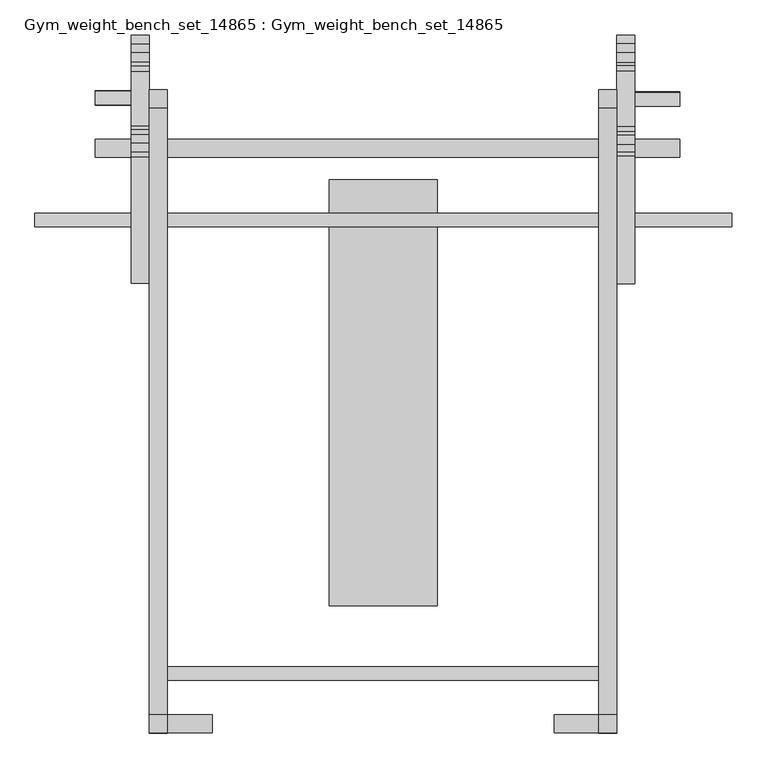
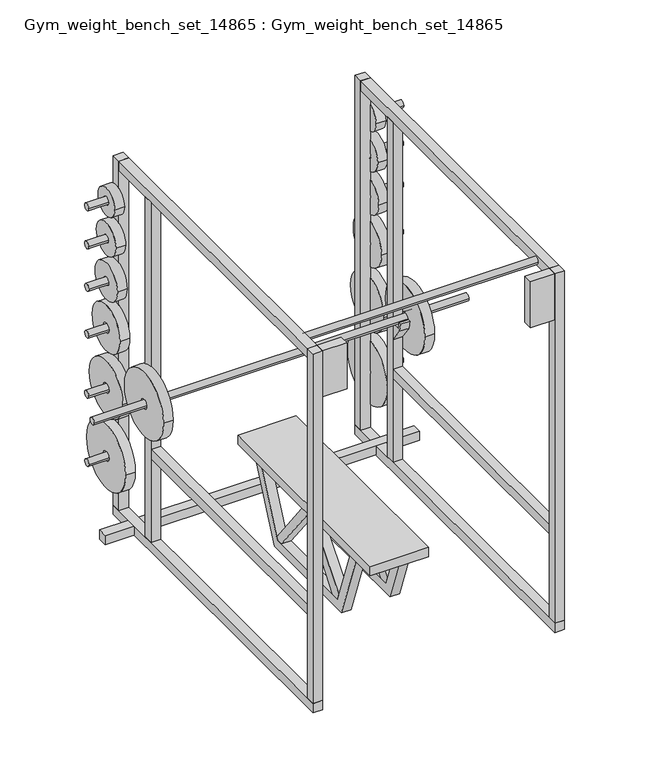
"""IFC4 building model written with IfcOpenShell, lengths in millimetres: furniture geometry, Gym_weight_bench_set_14865 : Gym_weight_bench_set_14865."""

from ifc_helpers import new_model, si_unit, point, frame, frame_2d, origin, place, context, project, spatial, polyline, circle_curve, trimmed, segment, composite_curve, outline, extrude, source, transform, mapped, element, save


def gym_weight_bench_set_14865_gym_weight_bench_set_14865_0f5544b4(model_context):
    return source(origin(), model_context, "Body", "SweptSolid", [
        extrude(outline(polyline([(0.0, 1816.1), (50.8, 1816.1), (50.8, 0.0), (0.0, 0.0), (0.0, 1816.1)])), frame((0.0, 0.0, 93.2100633), z_axis=(0.0, 0.0, 1.0), x_axis=(1.0, 0.0, 0.0)), (0.0, 0.0, 1.0), 50.8),
        extrude(outline(polyline([(0.0, 0.0), (0.0, 50.8), (50.8, 50.8), (50.8, 0.0), (0.0, 0.0)])), frame((0.0, 0.0, 144.0100633), z_axis=(0.0, 0.0, 1.0), x_axis=(1.0, 0.0, 0.0)), (0.0, 0.0, 1.0), 1938.7899367),
        extrude(outline(polyline([(0.0, 1473.2), (0.0, 1524.0), (50.8, 1524.0), (50.8, 1473.2), (0.0, 1473.2)])), frame((0.0, 0.0, 144.0100633), z_axis=(0.0, 0.0, 1.0), x_axis=(1.0, 0.0, 0.0)), (0.0, 0.0, 1.0), 1887.9899367),
        extrude(outline(polyline([(-152.4, 1676.4), (0.0, 1676.4), (50.8, 1676.4), (1270.0, 1676.4), (1498.6, 1676.4), (1498.6, 1625.6), (-152.4, 1625.6), (-152.4, 1676.4)])), frame((0.0, 0.0, 93.2100633), z_axis=(0.0, 0.0, 1.0), x_axis=(1.0, 0.0, 0.0)), (0.0, 0.0, 1.0), 50.8),
        extrude(outline(polyline([(1270.0, 1816.1), (1320.8, 1816.1), (1320.8, 0.0), (1270.0, 0.0), (1270.0, 1816.1)])), frame((0.0, 0.0, 93.2100633), z_axis=(0.0, 0.0, 1.0), x_axis=(1.0, 0.0, 0.0)), (0.0, 0.0, 1.0), 50.8),
        extrude(outline(polyline([(1270.0, 0.0), (1270.0, 50.8), (1320.8, 50.8), (1320.8, 0.0), (1270.0, 0.0)])), frame((0.0, 0.0, 144.0100633), z_axis=(0.0, 0.0, 1.0), x_axis=(1.0, 0.0, 0.0)), (0.0, 0.0, 1.0), 1938.7899367),
        extrude(outline(polyline([(1270.0, 1473.2), (1270.0, 1524.0), (1320.8, 1524.0), (1320.8, 1473.2), (1270.0, 1473.2)])), frame((0.0, 0.0, 144.0100633), z_axis=(0.0, 0.0, 1.0), x_axis=(1.0, 0.0, 0.0)), (0.0, 0.0, 1.0), 1887.9899367),
        extrude(outline(polyline([(0.0, 1765.3), (0.0, 1816.1), (50.8, 1816.1), (50.8, 1765.3), (0.0, 1765.3)])), frame((0.0, 0.0, 144.0100633), z_axis=(0.0, 0.0, 1.0), x_axis=(1.0, 0.0, 0.0)), (0.0, 0.0, 1.0), 1938.7899367),
        extrude(outline(polyline([(1270.0, 1765.3), (1270.0, 1816.1), (1320.8, 1816.1), (1320.8, 1765.3), (1270.0, 1765.3)])), frame((0.0, 0.0, 144.0100633), z_axis=(0.0, 0.0, 1.0), x_axis=(1.0, 0.0, 0.0)), (0.0, 0.0, 1.0), 1938.7899367),
        extrude(outline(polyline([(0.0, 50.8), (0.0, 1816.1), (50.8, 1816.1), (50.8, 50.8), (0.0, 50.8)])), frame((0.0, 0.0, 2032.0), z_axis=(0.0, 0.0, 1.0), x_axis=(1.0, 0.0, 0.0)), (0.0, 0.0, 1.0), 50.8),
        extrude(outline(polyline([(1270.0, 50.8), (1270.0, 1816.1), (1320.8, 1816.1), (1320.8, 50.8), (1270.0, 50.8)])), frame((0.0, 0.0, 2032.0), z_axis=(0.0, 0.0, 1.0), x_axis=(1.0, 0.0, 0.0)), (0.0, 0.0, 1.0), 50.8),
        extrude(outline(polyline([(0.0, 50.8), (0.0, 1473.2), (50.8, 1473.2), (50.8, 50.8), (0.0, 50.8)])), frame((0.0, 0.0, 609.6), z_axis=(0.0, 0.0, 1.0), x_axis=(1.0, 0.0, 0.0)), (0.0, 0.0, 1.0), 50.8),
        extrude(outline(polyline([(1270.0, 50.8), (1270.0, 1473.2), (1320.8, 1473.2), (1320.8, 50.8), (1270.0, 50.8)])), frame((0.0, 0.0, 609.6), z_axis=(0.0, 0.0, 1.0), x_axis=(1.0, 0.0, 0.0)), (0.0, 0.0, 1.0), 50.8),
        extrude(outline(composite_curve([segment(trimmed(circle_curve(frame_2d((168.0556142, 2057.8602895)), 19.05), [point((149.0056142, 2057.8602895))], [point((187.1056142, 2057.8602895))], False, "CARTESIAN"), True, "CONTINUOUS"), segment(trimmed(circle_curve(frame_2d((168.0556142, 2057.8602895)), 19.05), [point((187.1056142, 2057.8602895))], [point((149.0056142, 2057.8602895))], False, "CARTESIAN"), True, "CONTINUOUS")], self_intersect=False)), frame((50.8, 0.0, 0.0), z_axis=(1.0, 0.0, 0.0), x_axis=(0.0, 1.0, 0.0)), (0.0, 0.0, 1.0), 1219.2),
        extrude(outline(composite_curve([segment(trimmed(circle_curve(frame_2d((1791.2245511, 448.53524)), 19.05), [point((1772.1745511, 448.53524))], [point((1810.2745511, 448.53524))], False, "CARTESIAN"), True, "CONTINUOUS"), segment(trimmed(circle_curve(frame_2d((1791.2245511, 448.53524)), 19.05), [point((1810.2745511, 448.53524))], [point((1772.1745511, 448.53524))], False, "CARTESIAN"), True, "CONTINUOUS")], self_intersect=False)), frame((-152.4, 0.0, 0.0), z_axis=(1.0, 0.0, 0.0), x_axis=(0.0, 1.0, 0.0)), (0.0, 0.0, 1.0), 152.4),
        extrude(outline(composite_curve([segment(trimmed(circle_curve(frame_2d((1792.8120511, 826.36024)), 19.05), [point((1773.7620511, 826.36024))], [point((1811.8620511, 826.36024))], False, "CARTESIAN"), True, "CONTINUOUS"), segment(trimmed(circle_curve(frame_2d((1792.8120511, 826.36024)), 19.05), [point((1811.8620511, 826.36024))], [point((1773.7620511, 826.36024))], False, "CARTESIAN"), True, "CONTINUOUS")], self_intersect=False)), frame((-152.4, 0.0, 0.0), z_axis=(1.0, 0.0, 0.0), x_axis=(0.0, 1.0, 0.0)), (0.0, 0.0, 1.0), 152.4),
        extrude(outline(composite_curve([segment(trimmed(circle_curve(frame_2d((1792.4151761, 1865.775865)), 19.05), [point((1773.3651761, 1865.775865))], [point((1811.4651761, 1865.775865))], False, "CARTESIAN"), True, "CONTINUOUS"), segment(trimmed(circle_curve(frame_2d((1792.4151761, 1865.775865)), 19.05), [point((1811.4651761, 1865.775865))], [point((1773.3651761, 1865.775865))], False, "CARTESIAN"), True, "CONTINUOUS")], self_intersect=False)), frame((-152.4, 0.0, 0.0), z_axis=(1.0, 0.0, 0.0), x_axis=(0.0, 1.0, 0.0)), (0.0, 0.0, 1.0), 152.4),
        extrude(outline(composite_curve([segment(trimmed(circle_curve(frame_2d((1793.6058011, 1654.24149)), 19.05), [point((1774.5558011, 1654.24149))], [point((1812.6558011, 1654.24149))], False, "CARTESIAN"), True, "CONTINUOUS"), segment(trimmed(circle_curve(frame_2d((1793.6058011, 1654.24149)), 19.05), [point((1812.6558011, 1654.24149))], [point((1774.5558011, 1654.24149))], False, "CARTESIAN"), True, "CONTINUOUS")], self_intersect=False)), frame((-152.4, 0.0, 0.0), z_axis=(1.0, 0.0, 0.0), x_axis=(0.0, 1.0, 0.0)), (0.0, 0.0, 1.0), 152.4),
        extrude(outline(composite_curve([segment(trimmed(circle_curve(frame_2d((1791.2245511, 1420.08524)), 19.05), [point((1772.1745511, 1420.08524))], [point((1810.2745511, 1420.08524))], False, "CARTESIAN"), True, "CONTINUOUS"), segment(trimmed(circle_curve(frame_2d((1791.2245511, 1420.08524)), 19.05), [point((1810.2745511, 1420.08524))], [point((1772.1745511, 1420.08524))], False, "CARTESIAN"), True, "CONTINUOUS")], self_intersect=False)), frame((-152.4, 0.0, 0.0), z_axis=(1.0, 0.0, 0.0), x_axis=(0.0, 1.0, 0.0)), (0.0, 0.0, 1.0), 152.4),
        extrude(outline(composite_curve([segment(trimmed(circle_curve(frame_2d((1792.0183011, 1159.73524)), 19.05), [point((1772.9683011, 1159.73524))], [point((1811.0683011, 1159.73524))], False, "CARTESIAN"), True, "CONTINUOUS"), segment(trimmed(circle_curve(frame_2d((1792.0183011, 1159.73524)), 19.05), [point((1811.0683011, 1159.73524))], [point((1772.9683011, 1159.73524))], False, "CARTESIAN"), True, "CONTINUOUS")], self_intersect=False)), frame((-152.4, 0.0, 0.0), z_axis=(1.0, 0.0, 0.0), x_axis=(0.0, 1.0, 0.0)), (0.0, 0.0, 1.0), 152.4),
        extrude(outline(composite_curve([segment(trimmed(circle_curve(frame_2d((1788.3835299, 1862.6771224)), 19.05), [point((1769.3335299, 1862.6771224))], [point((1807.4335299, 1862.6771224))], False, "CARTESIAN"), True, "CONTINUOUS"), segment(trimmed(circle_curve(frame_2d((1788.3835299, 1862.6771224)), 19.05), [point((1807.4335299, 1862.6771224))], [point((1769.3335299, 1862.6771224))], False, "CARTESIAN"), True, "CONTINUOUS")], self_intersect=False)), frame((1320.8, 0.0, 0.0), z_axis=(1.0, 0.0, 0.0), x_axis=(0.0, 1.0, 0.0)), (0.0, 0.0, 1.0), 177.8),
        extrude(outline(composite_curve([segment(trimmed(circle_curve(frame_2d((1789.9710299, 1650.9298353)), 19.05), [point((1770.9210299, 1650.9298353))], [point((1809.0210299, 1650.9298353))], False, "CARTESIAN"), True, "CONTINUOUS"), segment(trimmed(circle_curve(frame_2d((1789.9710299, 1650.9298353)), 19.05), [point((1809.0210299, 1650.9298353))], [point((1770.9210299, 1650.9298353))], False, "CARTESIAN"), True, "CONTINUOUS")], self_intersect=False)), frame((1320.8, 0.0, 0.0), z_axis=(1.0, 0.0, 0.0), x_axis=(0.0, 1.0, 0.0)), (0.0, 0.0, 1.0), 177.8),
        extrude(outline(composite_curve([segment(trimmed(circle_curve(frame_2d((1789.9710299, 1422.3298353)), 19.05), [point((1770.9210299, 1422.3298353))], [point((1809.0210299, 1422.3298353))], False, "CARTESIAN"), True, "CONTINUOUS"), segment(trimmed(circle_curve(frame_2d((1789.9710299, 1422.3298353)), 19.05), [point((1809.0210299, 1422.3298353))], [point((1770.9210299, 1422.3298353))], False, "CARTESIAN"), True, "CONTINUOUS")], self_intersect=False)), frame((1320.8, 0.0, 0.0), z_axis=(1.0, 0.0, 0.0), x_axis=(0.0, 1.0, 0.0)), (0.0, 0.0, 1.0), 177.8),
        extrude(outline(composite_curve([segment(trimmed(circle_curve(frame_2d((1789.9710299, 1160.2424636)), 19.05), [point((1770.9210299, 1160.2424636))], [point((1809.0210299, 1160.2424636))], False, "CARTESIAN"), True, "CONTINUOUS"), segment(trimmed(circle_curve(frame_2d((1789.9710299, 1160.2424636)), 19.05), [point((1809.0210299, 1160.2424636))], [point((1770.9210299, 1160.2424636))], False, "CARTESIAN"), True, "CONTINUOUS")], self_intersect=False)), frame((1320.8, 0.0, 0.0), z_axis=(1.0, 0.0, 0.0), x_axis=(0.0, 1.0, 0.0)), (0.0, 0.0, 1.0), 177.8),
        extrude(outline(composite_curve([segment(trimmed(circle_curve(frame_2d((1791.5585299, 826.8674636)), 19.05), [point((1772.5085299, 826.8674636))], [point((1810.6085299, 826.8674636))], False, "CARTESIAN"), True, "CONTINUOUS"), segment(trimmed(circle_curve(frame_2d((1791.5585299, 826.8674636)), 19.05), [point((1810.6085299, 826.8674636))], [point((1772.5085299, 826.8674636))], False, "CARTESIAN"), True, "CONTINUOUS")], self_intersect=False)), frame((1320.8, 0.0, 0.0), z_axis=(1.0, 0.0, 0.0), x_axis=(0.0, 1.0, 0.0)), (0.0, 0.0, 1.0), 177.8),
        extrude(outline(composite_curve([segment(trimmed(circle_curve(frame_2d((1789.9710299, 448.917051)), 19.05), [point((1770.9210299, 448.917051))], [point((1809.0210299, 448.917051))], False, "CARTESIAN"), True, "CONTINUOUS"), segment(trimmed(circle_curve(frame_2d((1789.9710299, 448.917051)), 19.05), [point((1809.0210299, 448.917051))], [point((1770.9210299, 448.917051))], False, "CARTESIAN"), True, "CONTINUOUS")], self_intersect=False)), frame((1320.8, 0.0, 0.0), z_axis=(1.0, 0.0, 0.0), x_axis=(0.0, 1.0, 0.0)), (0.0, 0.0, 1.0), 177.8),
        extrude(outline(polyline([(177.8, 0.0), (50.8, 0.0), (50.8, 50.8), (177.8, 50.8), (177.8, 0.0)])), frame((0.0, 0.0, 1828.8), z_axis=(0.0, 0.0, 1.0), x_axis=(1.0, 0.0, 0.0)), (0.0, 0.0, 1.0), 254.0),
        extrude(outline(polyline([(1270.0, 0.0), (1143.0, 0.0), (1143.0, 50.8), (1270.0, 50.8), (1270.0, 0.0)])), frame((0.0, 0.0, 1828.8), z_axis=(0.0, 0.0, 1.0), x_axis=(1.0, 0.0, 0.0)), (0.0, 0.0, 1.0), 254.0),
        extrude(outline(composite_curve([segment(trimmed(circle_curve(frame_2d((1448.5134797, 945.953956)), 19.05), [point((1429.4634797, 945.953956))], [point((1467.5634797, 945.953956))], False, "CARTESIAN"), True, "CONTINUOUS"), segment(trimmed(circle_curve(frame_2d((1448.5134797, 945.953956)), 19.05), [point((1467.5634797, 945.953956))], [point((1429.4634797, 945.953956))], False, "CARTESIAN"), True, "CONTINUOUS")], self_intersect=False)), frame((-322.3423226, 0.0, 0.0), z_axis=(1.0, 0.0, 0.0), x_axis=(0.0, 1.0, 0.0)), (0.0, 0.0, 1.0), 1966.9449532),
        extrude(outline(polyline([(1422.4, 920.0682148), (1473.2, 920.0682148), (1473.2, 823.1962833), (1411.9053319, 907.5611564), (1404.1016184, 951.8182148), (1416.8016184, 951.8182148), (1422.4, 920.0682148)])), frame((0.0, 0.0, 0.0), z_axis=(1.0, 0.0, 0.0), x_axis=(0.0, 1.0, 0.0)), (0.0, 0.0, 1.0), 50.8),
        extrude(outline(polyline([(1422.4, 920.0682148), (1473.2, 920.0682148), (1473.2, 823.1962833), (1411.9053319, 907.5611564), (1404.1016184, 951.8182148), (1416.8016184, 951.8182148), (1422.4, 920.0682148)])), frame((1270.0, 0.0, 0.0), z_axis=(1.0, 0.0, 0.0), x_axis=(0.0, 1.0, 0.0)), (0.0, 0.0, 1.0), 50.8),
        extrude(outline(composite_curve([segment(trimmed(circle_curve(frame_2d((1792.6730331, 448.4299911)), 177.8), [point((1614.8730331, 448.4299911))], [point((1970.4730331, 448.4299911))], False, "CARTESIAN"), True, "CONTINUOUS"), segment(trimmed(circle_curve(frame_2d((1792.6730331, 448.4299911)), 177.8), [point((1970.4730331, 448.4299911))], [point((1614.8730331, 448.4299911))], False, "CARTESIAN"), True, "CONTINUOUS")], self_intersect=False), holes=[composite_curve([segment(trimmed(circle_curve(frame_2d((1792.6730331, 448.4299911)), 25.7855331), [point((1766.8875, 448.4299911))], [point((1818.4585662, 448.4299911))], True, "CARTESIAN"), True, "CONTINUOUS"), segment(trimmed(circle_curve(frame_2d((1792.6730331, 448.4299911)), 25.7855331), [point((1818.4585662, 448.4299911))], [point((1766.8875, 448.4299911))], True, "CARTESIAN"), True, "CONTINUOUS")], self_intersect=False)]), frame((-50.8, 0.0, 0.0), z_axis=(1.0, 0.0, 0.0), x_axis=(0.0, 1.0, 0.0)), (0.0, 0.0, 1.0), 50.8),
        extrude(outline(composite_curve([segment(trimmed(circle_curve(frame_2d((1792.6730331, 826.2549911)), 152.4), [point((1640.2730331, 826.2549911))], [point((1945.0730331, 826.2549911))], False, "CARTESIAN"), True, "CONTINUOUS"), segment(trimmed(circle_curve(frame_2d((1792.6730331, 826.2549911)), 152.4), [point((1945.0730331, 826.2549911))], [point((1640.2730331, 826.2549911))], False, "CARTESIAN"), True, "CONTINUOUS")], self_intersect=False), holes=[composite_curve([segment(trimmed(circle_curve(frame_2d((1792.6730331, 826.2549911)), 25.7855331), [point((1766.8875, 826.2549911))], [point((1818.4585662, 826.2549911))], True, "CARTESIAN"), True, "CONTINUOUS"), segment(trimmed(circle_curve(frame_2d((1792.6730331, 826.2549911)), 25.7855331), [point((1818.4585662, 826.2549911))], [point((1766.8875, 826.2549911))], True, "CARTESIAN"), True, "CONTINUOUS")], self_intersect=False)]), frame((-50.8, 0.0, 0.0), z_axis=(1.0, 0.0, 0.0), x_axis=(0.0, 1.0, 0.0)), (0.0, 0.0, 1.0), 50.8),
        extrude(outline(composite_curve([segment(trimmed(circle_curve(frame_2d((1792.6730331, 1159.6299911)), 127.0), [point((1665.6730331, 1159.6299911))], [point((1919.6730331, 1159.6299911))], False, "CARTESIAN"), True, "CONTINUOUS"), segment(trimmed(circle_curve(frame_2d((1792.6730331, 1159.6299911)), 127.0), [point((1919.6730331, 1159.6299911))], [point((1665.6730331, 1159.6299911))], False, "CARTESIAN"), True, "CONTINUOUS")], self_intersect=False), holes=[composite_curve([segment(trimmed(circle_curve(frame_2d((1792.6730331, 1159.6299911)), 25.7855331), [point((1766.8875, 1159.6299911))], [point((1818.4585662, 1159.6299911))], True, "CARTESIAN"), True, "CONTINUOUS"), segment(trimmed(circle_curve(frame_2d((1792.6730331, 1159.6299911)), 25.7855331), [point((1818.4585662, 1159.6299911))], [point((1766.8875, 1159.6299911))], True, "CARTESIAN"), True, "CONTINUOUS")], self_intersect=False)]), frame((-50.8, 0.0, 0.0), z_axis=(1.0, 0.0, 0.0), x_axis=(0.0, 1.0, 0.0)), (0.0, 0.0, 1.0), 50.8),
        extrude(outline(composite_curve([segment(trimmed(circle_curve(frame_2d((1448.1855331, 945.5372652)), 177.8), [point((1270.3855331, 945.5372652))], [point((1625.9855331, 945.5372652))], False, "CARTESIAN"), True, "CONTINUOUS"), segment(trimmed(circle_curve(frame_2d((1448.1855331, 945.5372652)), 177.8), [point((1625.9855331, 945.5372652))], [point((1270.3855331, 945.5372652))], False, "CARTESIAN"), True, "CONTINUOUS")], self_intersect=False), holes=[composite_curve([segment(trimmed(circle_curve(frame_2d((1448.1855331, 945.5372652)), 25.7855331), [point((1422.4, 945.5372652))], [point((1473.9710662, 945.5372652))], True, "CARTESIAN"), True, "CONTINUOUS"), segment(trimmed(circle_curve(frame_2d((1448.1855331, 945.5372652)), 25.7855331), [point((1473.9710662, 945.5372652))], [point((1422.4, 945.5372652))], True, "CARTESIAN"), True, "CONTINUOUS")], self_intersect=False)]), frame((-50.8, 0.0, 0.0), z_axis=(1.0, 0.0, 0.0), x_axis=(0.0, 1.0, 0.0)), (0.0, 0.0, 1.0), 50.8),
        extrude(outline(composite_curve([segment(trimmed(circle_curve(frame_2d((1790.3721267, 1859.8407645)), 76.2), [point((1714.1721267, 1859.8407645))], [point((1866.5721267, 1859.8407645))], False, "CARTESIAN"), True, "CONTINUOUS"), segment(trimmed(circle_curve(frame_2d((1790.3721267, 1859.8407645)), 76.2), [point((1866.5721267, 1859.8407645))], [point((1714.1721267, 1859.8407645))], False, "CARTESIAN"), True, "CONTINUOUS")], self_intersect=False), holes=[composite_curve([segment(trimmed(circle_curve(frame_2d((1792.2369373, 1865.5999932)), 21.4432675), [point((1770.7936698, 1865.5999932))], [point((1813.6802049, 1865.5999932))], True, "CARTESIAN"), True, "CONTINUOUS"), segment(trimmed(circle_curve(frame_2d((1792.2369373, 1865.5999932)), 21.4432675), [point((1813.6802049, 1865.5999932))], [point((1770.7936698, 1865.5999932))], True, "CARTESIAN"), True, "CONTINUOUS")], self_intersect=False)]), frame((-50.8, 0.0, 0.0), z_axis=(1.0, 0.0, 0.0), x_axis=(0.0, 1.0, 0.0)), (0.0, 0.0, 1.0), 50.8),
        extrude(outline(composite_curve([segment(trimmed(circle_curve(frame_2d((1792.64404, 1654.3866671)), 88.9), [point((1703.74404, 1654.3866671))], [point((1881.54404, 1654.3866671))], False, "CARTESIAN"), True, "CONTINUOUS"), segment(trimmed(circle_curve(frame_2d((1792.64404, 1654.3866671)), 88.9), [point((1881.54404, 1654.3866671))], [point((1703.74404, 1654.3866671))], False, "CARTESIAN"), True, "CONTINUOUS")], self_intersect=False), holes=[composite_curve([segment(trimmed(circle_curve(frame_2d((1792.64404, 1654.3866671)), 20.7181506), [point((1771.9258894, 1654.3866671))], [point((1813.3621906, 1654.3866671))], True, "CARTESIAN"), True, "CONTINUOUS"), segment(trimmed(circle_curve(frame_2d((1792.64404, 1654.3866671)), 20.7181506), [point((1813.3621906, 1654.3866671))], [point((1771.9258894, 1654.3866671))], True, "CARTESIAN"), True, "CONTINUOUS")], self_intersect=False)]), frame((-50.8, 0.0, 0.0), z_axis=(1.0, 0.0, 0.0), x_axis=(0.0, 1.0, 0.0)), (0.0, 0.0, 1.0), 50.8),
        extrude(outline(composite_curve([segment(trimmed(circle_curve(frame_2d((1791.2896953, 1420.0850266)), 101.6), [point((1689.6896953, 1420.0850266))], [point((1892.8896953, 1420.0850266))], False, "CARTESIAN"), True, "CONTINUOUS"), segment(trimmed(circle_curve(frame_2d((1791.2896953, 1420.0850266)), 101.6), [point((1892.8896953, 1420.0850266))], [point((1689.6896953, 1420.0850266))], False, "CARTESIAN"), True, "CONTINUOUS")], self_intersect=False), holes=[composite_curve([segment(trimmed(circle_curve(frame_2d((1791.2896953, 1420.0850266)), 21.3349156), [point((1769.9547796, 1420.0850266))], [point((1812.6246109, 1420.0850266))], True, "CARTESIAN"), True, "CONTINUOUS"), segment(trimmed(circle_curve(frame_2d((1791.2896953, 1420.0850266)), 21.3349156), [point((1812.6246109, 1420.0850266))], [point((1769.9547796, 1420.0850266))], True, "CARTESIAN"), True, "CONTINUOUS")], self_intersect=False)]), frame((-50.8, 0.0, 0.0), z_axis=(1.0, 0.0, 0.0), x_axis=(0.0, 1.0, 0.0)), (0.0, 0.0, 1.0), 50.8),
        extrude(outline(composite_curve([segment(trimmed(circle_curve(frame_2d((1791.0047799, 449.3731485)), 179.5423329), [point((1611.462447, 449.3731485))], [point((1970.5471128, 449.3731485))], False, "CARTESIAN"), True, "CONTINUOUS"), segment(trimmed(circle_curve(frame_2d((1791.0047799, 449.3731485)), 179.5423329), [point((1970.5471128, 449.3731485))], [point((1611.462447, 449.3731485))], False, "CARTESIAN"), True, "CONTINUOUS")], self_intersect=False), holes=[composite_curve([segment(trimmed(circle_curve(frame_2d((1791.0047799, 449.3731485)), 25.9804836), [point((1765.0242963, 449.3731485))], [point((1816.9852635, 449.3731485))], True, "CARTESIAN"), True, "CONTINUOUS"), segment(trimmed(circle_curve(frame_2d((1791.0047799, 449.3731485)), 25.9804836), [point((1816.9852635, 449.3731485))], [point((1765.0242963, 449.3731485))], True, "CARTESIAN"), True, "CONTINUOUS")], self_intersect=False)]), frame((1320.8, 0.0, 0.0), z_axis=(1.0, 0.0, 0.0), x_axis=(0.0, 1.0, 0.0)), (0.0, 0.0, 1.0), 50.8),
        extrude(outline(composite_curve([segment(trimmed(circle_curve(frame_2d((1448.1047799, 945.4668985)), 179.5423329), [point((1268.562447, 945.4668985))], [point((1627.6471128, 945.4668985))], False, "CARTESIAN"), True, "CONTINUOUS"), segment(trimmed(circle_curve(frame_2d((1448.1047799, 945.4668985)), 179.5423329), [point((1627.6471128, 945.4668985))], [point((1268.562447, 945.4668985))], False, "CARTESIAN"), True, "CONTINUOUS")], self_intersect=False), holes=[composite_curve([segment(trimmed(circle_curve(frame_2d((1448.1047799, 945.4668985)), 25.9804836), [point((1422.1242963, 945.4668985))], [point((1474.0852635, 945.4668985))], True, "CARTESIAN"), True, "CONTINUOUS"), segment(trimmed(circle_curve(frame_2d((1448.1047799, 945.4668985)), 25.9804836), [point((1474.0852635, 945.4668985))], [point((1422.1242963, 945.4668985))], True, "CARTESIAN"), True, "CONTINUOUS")], self_intersect=False)]), frame((1320.8, 0.0, 0.0), z_axis=(1.0, 0.0, 0.0), x_axis=(0.0, 1.0, 0.0)), (0.0, 0.0, 1.0), 50.8),
        extrude(outline(composite_curve([segment(trimmed(circle_curve(frame_2d((1792.7174395, 826.6813162)), 152.4), [point((1640.3174395, 826.6813162))], [point((1945.1174395, 826.6813162))], False, "CARTESIAN"), True, "CONTINUOUS"), segment(trimmed(circle_curve(frame_2d((1792.7174395, 826.6813162)), 152.4), [point((1945.1174395, 826.6813162))], [point((1640.3174395, 826.6813162))], False, "CARTESIAN"), True, "CONTINUOUS")], self_intersect=False), holes=[composite_curve([segment(trimmed(circle_curve(frame_2d((1792.7174395, 826.6813162)), 21.0651809), [point((1771.6522585, 826.6813162))], [point((1813.7826204, 826.6813162))], True, "CARTESIAN"), True, "CONTINUOUS"), segment(trimmed(circle_curve(frame_2d((1792.7174395, 826.6813162)), 21.0651809), [point((1813.7826204, 826.6813162))], [point((1771.6522585, 826.6813162))], True, "CARTESIAN"), True, "CONTINUOUS")], self_intersect=False)]), frame((1320.8, 0.0, 0.0), z_axis=(1.0, 0.0, 0.0), x_axis=(0.0, 1.0, 0.0)), (0.0, 0.0, 1.0), 50.8),
        extrude(outline(composite_curve([segment(trimmed(circle_curve(frame_2d((1790.9954276, 1161.3108664)), 128.7811923), [point((1662.2142353, 1161.3108664))], [point((1919.77662, 1161.3108664))], False, "CARTESIAN"), True, "CONTINUOUS"), segment(trimmed(circle_curve(frame_2d((1790.9954276, 1161.3108664)), 128.7811923), [point((1919.77662, 1161.3108664))], [point((1662.2142353, 1161.3108664))], False, "CARTESIAN"), True, "CONTINUOUS")], self_intersect=False), holes=[composite_curve([segment(trimmed(circle_curve(frame_2d((1790.9954276, 1161.3108664)), 25.4), [point((1765.5954276, 1161.3108664))], [point((1816.3954276, 1161.3108664))], True, "CARTESIAN"), True, "CONTINUOUS"), segment(trimmed(circle_curve(frame_2d((1790.9954276, 1161.3108664)), 25.4), [point((1816.3954276, 1161.3108664))], [point((1765.5954276, 1161.3108664))], True, "CARTESIAN"), True, "CONTINUOUS")], self_intersect=False)]), frame((1320.8, 0.0, 0.0), z_axis=(1.0, 0.0, 0.0), x_axis=(0.0, 1.0, 0.0)), (0.0, 0.0, 1.0), 50.8),
        extrude(outline(composite_curve([segment(trimmed(circle_curve(frame_2d((1791.0391205, 1422.0272209)), 101.6), [point((1689.4391205, 1422.0272209))], [point((1892.6391205, 1422.0272209))], False, "CARTESIAN"), True, "CONTINUOUS"), segment(trimmed(circle_curve(frame_2d((1791.0391205, 1422.0272209)), 101.6), [point((1892.6391205, 1422.0272209))], [point((1689.4391205, 1422.0272209))], False, "CARTESIAN"), True, "CONTINUOUS")], self_intersect=False), holes=[composite_curve([segment(trimmed(circle_curve(frame_2d((1791.0391205, 1422.0272209)), 25.4), [point((1765.6391205, 1422.0272209))], [point((1816.4391205, 1422.0272209))], True, "CARTESIAN"), True, "CONTINUOUS"), segment(trimmed(circle_curve(frame_2d((1791.0391205, 1422.0272209)), 25.4), [point((1816.4391205, 1422.0272209))], [point((1765.6391205, 1422.0272209))], True, "CARTESIAN"), True, "CONTINUOUS")], self_intersect=False)]), frame((1320.8, 0.0, 0.0), z_axis=(1.0, 0.0, 0.0), x_axis=(0.0, 1.0, 0.0)), (0.0, 0.0, 1.0), 50.8),
        extrude(outline(composite_curve([segment(trimmed(circle_curve(frame_2d((1790.6727551, 1651.4179067)), 92.5921988), [point((1698.0805563, 1651.4179067))], [point((1883.2649539, 1651.4179067))], False, "CARTESIAN"), True, "CONTINUOUS"), segment(trimmed(circle_curve(frame_2d((1790.6727551, 1651.4179067)), 92.5921988), [point((1883.2649539, 1651.4179067))], [point((1698.0805563, 1651.4179067))], False, "CARTESIAN"), True, "CONTINUOUS")], self_intersect=False), holes=[composite_curve([segment(trimmed(circle_curve(frame_2d((1790.6727551, 1651.4179067)), 25.4), [point((1765.2727551, 1651.4179067))], [point((1816.0727551, 1651.4179067))], True, "CARTESIAN"), True, "CONTINUOUS"), segment(trimmed(circle_curve(frame_2d((1790.6727551, 1651.4179067)), 25.4), [point((1816.0727551, 1651.4179067))], [point((1765.2727551, 1651.4179067))], True, "CARTESIAN"), True, "CONTINUOUS")], self_intersect=False)]), frame((1320.8, 0.0, 0.0), z_axis=(1.0, 0.0, 0.0), x_axis=(0.0, 1.0, 0.0)), (0.0, 0.0, 1.0), 50.8),
        extrude(outline(composite_curve([segment(trimmed(circle_curve(frame_2d((1790.2300174, 1859.1377235)), 78.035269), [point((1712.1947484, 1859.1377235))], [point((1868.2652864, 1859.1377235))], False, "CARTESIAN"), True, "CONTINUOUS"), segment(trimmed(circle_curve(frame_2d((1790.2300174, 1859.1377235)), 78.035269), [point((1868.2652864, 1859.1377235))], [point((1712.1947484, 1859.1377235))], False, "CARTESIAN"), True, "CONTINUOUS")], self_intersect=False), holes=[composite_curve([segment(trimmed(circle_curve(frame_2d((1789.4362674, 1861.5189735)), 19.05), [point((1770.3862674, 1861.5189735))], [point((1808.4862674, 1861.5189735))], True, "CARTESIAN"), True, "CONTINUOUS"), segment(trimmed(circle_curve(frame_2d((1789.4362674, 1861.5189735)), 19.05), [point((1808.4862674, 1861.5189735))], [point((1770.3862674, 1861.5189735))], True, "CARTESIAN"), True, "CONTINUOUS")], self_intersect=False)]), frame((1320.8, 0.0, 0.0), z_axis=(1.0, 0.0, 0.0), x_axis=(0.0, 1.0, 0.0)), (0.0, 0.0, 1.0), 50.8),
        extrude(outline(polyline([(812.8, 1562.1), (812.8, 359.327771), (508.0, 359.327771), (508.0, 1562.1), (812.8, 1562.1)])), frame((0.0, 0.0, 457.2), z_axis=(0.0, 0.0, 1.0), x_axis=(1.0, 0.0, 0.0)), (0.0, 0.0, 1.0), 50.8),
        extrude(outline(polyline([(621.4315025, 93.2100633), (488.95, 457.2), (543.0102308, 457.2), (657.0020455, 144.0100633), (1202.8491197, 144.0100633), (1342.2902635, 457.2), (1393.0902635, 457.2), (1231.0315025, 93.2100633), (621.4315025, 93.2100633)])), frame((508.0, 0.0, 0.0), z_axis=(1.0, 0.0, 0.0), x_axis=(0.0, 1.0, 0.0)), (0.0, 0.0, 1.0), 50.8),
        extrude(outline(polyline([(978.5428756, 455.1600633), (1212.237329, 153.3982726), (1202.8491197, 144.0100633), (1166.8576142, 144.0100633), (925.8926166, 455.1600633), (978.5428756, 455.1600633)])), frame((508.0, 0.0, 0.0), z_axis=(1.0, 0.0, 0.0), x_axis=(0.0, 1.0, 0.0)), (0.0, 0.0, 1.0), 50.8),
        extrude(outline(polyline([(657.0020455, 144.0100633), (643.1994997, 181.9322462), (874.1765704, 457.2), (929.9255826, 457.2), (929.9255826, 444.5), (695.1571142, 144.0100633), (657.0020455, 144.0100633)])), frame((508.0, 0.0, 0.0), z_axis=(1.0, 0.0, 0.0), x_axis=(0.0, 1.0, 0.0)), (0.0, 0.0, 1.0), 50.8),
        extrude(outline(polyline([(621.4315025, 93.2100633), (488.95, 457.2), (543.0102308, 457.2), (657.0020455, 144.0100633), (1202.8491197, 144.0100633), (1342.2902635, 457.2), (1393.0902635, 457.2), (1231.0315025, 93.2100633), (621.4315025, 93.2100633)])), frame((762.0, 0.0, 0.0), z_axis=(1.0, 0.0, 0.0), x_axis=(0.0, 1.0, 0.0)), (0.0, 0.0, 1.0), 50.8),
        extrude(outline(polyline([(978.5428756, 455.1600633), (1212.237329, 153.3982726), (1202.8491197, 144.0100633), (1166.8576142, 144.0100633), (925.8926166, 455.1600633), (978.5428756, 455.1600633)])), frame((762.0, 0.0, 0.0), z_axis=(1.0, 0.0, 0.0), x_axis=(0.0, 1.0, 0.0)), (0.0, 0.0, 1.0), 50.8),
        extrude(outline(polyline([(657.0020455, 144.0100633), (643.1994997, 181.9322462), (874.1765704, 457.2), (929.9255826, 457.2), (929.9255826, 444.5), (695.1571142, 144.0100633), (657.0020455, 144.0100633)])), frame((762.0, 0.0, 0.0), z_axis=(1.0, 0.0, 0.0), x_axis=(0.0, 1.0, 0.0)), (0.0, 0.0, 1.0), 50.8),
    ])


if __name__ == "__main__":
    model = new_model("IFC4")
    model_context = context("Model", 3, world=origin())
    ifc_project = project(units=[si_unit("LENGTHUNIT", "METRE", prefix="MILLI")], contexts=[model_context])
    site = spatial("IfcSite", under=ifc_project)
    building = spatial("IfcBuilding", under=site)
    placement = place(None, origin())
    gym_weight_bench_set_14865_gym_weight_bench_set_14865_shape = gym_weight_bench_set_14865_gym_weight_bench_set_14865_0f5544b4(model_context)
    element("IfcFurniture", 1, ObjectType="Gym_weight_bench_set_14865 : Gym_weight_bench_set_14865", at=placement, inside=building, context=model_context, shape_type="MappedRepresentation", body=[
        mapped(gym_weight_bench_set_14865_gym_weight_bench_set_14865_shape, transform((0.0, 0.0, 0.0), x_axis=(1.0, 0.0, 0.0), y_axis=(0.0, 1.0, 0.0), z_axis=(0.0, 0.0, 1.0))),
    ])
    save(model, "model.ifc")

# Revit data of these elements
# Type "Gym_weight_bench_set_14865 : Gym_weight_bench_set_14865"
#   Default Elevation = 0
# Element 1 (IfcFurniture, "Gym_weight_bench_set_14865 : Gym_weight_bench_set_14865")
#   Materials on its faces: "black", "silver", "white"
# Materials
#   "black": class "Metal", colour RGB 0 0 0, transparency 0
#   "silver": class "Generic", colour RGB 120 120 120, transparency 0, Cost = 0
#   "white": class "Generic", colour RGB 120 120 120, transparency 0, Cost = 0
